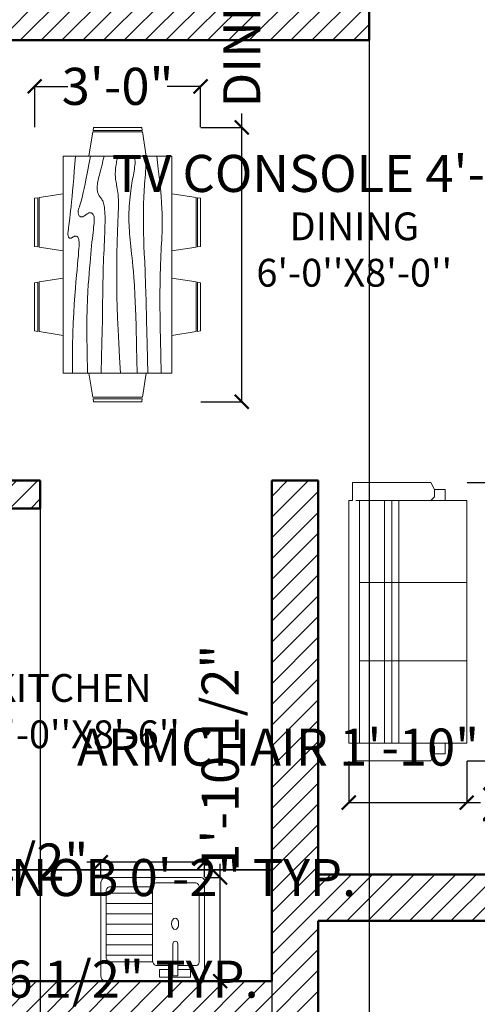
# Model space of a CAD drawing. Units: inches. Extents: x 1945 to 2401, y 1770 to 2289.
# Tile 3 of 5: x 2078 to 2177, y 1893 to 2105. Entities that reach past the tile are written whole.
import ezdxf

# ---------------------------------------------------------------- set-up
doc = ezdxf.new("R2010")
doc.units = ezdxf.units.IN
for name, color, linetype, lineweight in [('A-ANNO-DIMS', 2, 'Continuous', 18), ('A-AREA-IDEN', 7, 'Continuous', 25), ('A-FLOR-FIXT', 9, 'Continuous', 18), ('A-WALL-PATT', 8, 'Continuous', 13), ('B-FURNITURE', 22, 'Continuous', 18), ('kitchen', 122, 'Continuous', 25), ('Walls', 7, 'Continuous', 50)]:
    doc.layers.add(name, color=color, linetype=linetype, lineweight=lineweight)
doc.styles.get("Standard").update_dxf_attribs({"font": 'arial.ttf'})
doc.dimstyles.get("Standard").update_dxf_attribs({"dimtxt": 8, "dimasz": 3, "dimexe": 0.18, "dimexo": 0.0625, "dimgap": 0.09, "dimtad": 0, "dimdec": 1, "dimzin": 0, "dimdsep": 46, "dimlunit": 4, "dimtxsty": 'Standard', "dimblk": 'ARCHTICK', "dimcen": 0.09, "dimadec": 0, "dimazin": 0, "dimtfac": 1, "dimtdec": 1, "dimtofl": 0, "dimtmove": 0, "dimatfit": 3, "dimfxl": 1, "dimtolj": 1, "dimtzin": 0, "dimarcsym": 0})

# ---------------------------------------------------------------- blocks, each defined once
blk = doc.blocks.new('12PCOU13')
at = {"color": 0, "linetype": 'ByBlock'}
for p, q in [((24, 37), (24, 35)), ((23, 34), (2, 34)), ((3, -34), (3, 34)), ((10, 34), (10, -34)), ((12, 34), (12, -34)), ((14, 34), (14, -34)), ((24, 35), (23, 34)), ((27, 34), (23, 34)), ((33, 11), (3, 11)), ((33, -11), (3, -11)), ((23, -34), (2, -34)), ((27, -34), (23, -34)), ((24, -35), (23, -34)), ((24, -37), (24, -35))]:
    blk.add_line(p, q, dxfattribs=at)
blk.add_lwpolyline([(1, -39), (1, -34), (0, -34), (0, 34), (1, 34), (1, 39), (23, 39), (24, 37), (27, 37), (27, 34), (33, 34), (33, -34), (27, -34), (27, -37), (24, -37), (23, -39)], close=True, dxfattribs=at)
blk = doc.blocks.new('Dining Set - 36 x 72 in.')
for p, q in [((-22, 27.5), (-22.1562, 26.50042)), ((-5.8416, 26.5), (-22.1534, 26.5)), ((-22, 27.5), (-6, 27.5)), ((-5.8437, 26.49966), (-6, 27.5)), ((6, 27.5), (5.8438, 26.50042)), ((22.1584, 26.5), (5.8466, 26.5)), ((6, 27.5), (22, 27.5)), ((22.1563, 26.49966), (22, 27.5)), ((-22.2343, 26.00059), (-23.4847, 17.99762)), ((-22.2304, 26), (-5.7608, 26)), ((-4.5152, 17.99762), (-5.7655, 25.99926)), ((5.7657, 26.00059), (4.5153, 17.99762)), ((5.7696, 26), (22.2392, 26)), ((23.4848, 17.99762), (22.2345, 25.99926)), ((36, 18), (-36, 18)), ((-36, 18), (-36, -18)), ((36, -18), (36, 18)), ((-45.5, 8), (-44.5004, 8.15617)), ((-45.5, 8), (-45.5, -8)), ((-44.5, -8.15843), (-44.5, 8.15338)), ((-44.0006, 8.23428), (-35.9976, 9.48474)), ((-44, 8.23041), (-44, -8.23915)), ((44.0006, 8.23428), (35.9976, 9.48474)), ((44, 8.23041), (44, -8.23915)), ((44.5, -8.15843), (44.5, 8.15338)), ((45.5, 8), (44.5005, 8.15617)), ((45.5, 8), (45.5, -8)), ((-44.4997, -8.15631), (-45.5, -8)), ((-35.9976, -9.48476), (-43.9993, -8.2345)), ((35.9976, -9.48476), (43.9993, -8.2345)), ((44.4997, -8.15631), (45.5, -8)), ((-36, -18), (36, -18)), ((-22.2343, -26.0006), (-23.4847, -17.99762)), ((-4.5152, -17.99762), (-5.7655, -25.99928)), ((5.7657, -26.0006), (4.5153, -17.99762)), ((23.4848, -17.99762), (22.2345, -25.99928)), ((-22.2304, -26), (-5.7608, -26)), ((5.7696, -26), (22.2392, -26)), ((-22, -27.5), (-22.1562, -26.50044)), ((-5.8416, -26.5), (-22.1534, -26.5)), ((-22, -27.5), (-6, -27.5)), ((-5.8437, -26.49967), (-6, -27.5)), ((6, -27.5), (5.8438, -26.50044)), ((22.1584, -26.5), (5.8466, -26.5)), ((6, -27.5), (22, -27.5)), ((22.1563, -26.49967), (22, -27.5))]:
    blk.add_line(p, q)
for points in [[(-36, 15), (-31.1772, 14.97754), (-26.8079, 14.91406), (-22.8538, 14.81543), (-19.276, 14.6875), (-16.0362, 14.53613), (-13.0957, 14.36718), (-10.4159, 14.18652), (-7.9583, 14), (-5.6904, 13.81315), (-3.6035, 13.63021), (-1.6954, 13.45508), (0.0365, 13.29166), (1.5945, 13.14388), (2.9811, 13.01562), (4.1988, 12.9108), (5.25, 12.83333), (6.1393, 12.78613), (6.8802, 12.76823), (7.4883, 12.77767), (7.9792, 12.8125), (8.3685, 12.87077), (8.6719, 12.95052), (8.9049, 13.0498), (9.0833, 13.16666), (9.2205, 13.29899), (9.3216, 13.44401), (9.3895, 13.59879), (9.4271, 13.76041), (9.4373, 13.92594), (9.4232, 14.09245), (9.3875, 14.257), (9.3333, 14.41666), (9.2638, 14.56917), (9.1836, 14.71484), (9.0975, 14.85465), (9.0104, 14.98958), (8.9272, 15.1206), (8.8529, 15.2487), (8.7922, 15.37483), (8.75, 15.5), (8.7305, 15.62467), (8.7344, 15.74739), (8.7617, 15.86621), (8.8125, 15.97916), (8.8867, 16.08431), (8.9844, 16.17968), (9.1055, 16.26334), (9.25, 16.33333), (9.4189, 16.38802), (9.6172, 16.42708), (9.8506, 16.45052), (10.125, 16.45833), (10.4463, 16.45052), (10.8203, 16.42708), (11.2529, 16.38802), (11.75, 16.33333), (12.3184, 16.26318), (12.9694, 16.17838), (13.7151, 16.07991), (14.5677, 15.96875), (15.5395, 15.84586), (16.6426, 15.71224), (17.8893, 15.56884), (19.2917, 15.41666), (20.859, 15.25667), (22.5879, 15.08984), (24.4721, 14.91715), (26.5052, 14.73958), (28.6809, 14.5581), (30.9929, 14.3737), (33.4347, 14.18733), (36, 14)], [(-36, 10), (-28.9766, 10.14274), (-23.1725, 10.20442), (-18.4241, 10.19775), (-14.5677, 10.13541), (-11.4399, 10.03011), (-8.877, 9.89453), (-6.7154, 9.74137), (-4.7917, 9.58333), (-2.9698, 9.43082), (-1.2246, 9.28515), (0.4415, 9.14534), (2.026, 9.01041), (3.5266, 8.87939), (4.9408, 8.7513), (6.266, 8.62516), (7.5, 8.5), (8.6411, 8.37549), (9.6914, 8.2539), (10.6538, 8.13818), (11.5312, 8.03125), (12.3267, 7.93603), (13.043, 7.85547), (13.6831, 7.79248), (14.25, 7.75), (14.7471, 7.7303), (15.1797, 7.73307), (15.5537, 7.75732), (15.875, 7.80208), (16.1494, 7.86637), (16.3828, 7.94922), (16.5811, 8.04964), (16.75, 8.16666), (16.8944, 8.29915), (17.0143, 8.44531), (17.1089, 8.60319), (17.1771, 8.77083), (17.218, 8.94629), (17.2305, 9.1276), (17.2137, 9.31282), (17.1667, 9.5), (17.0895, 9.6875), (16.987, 9.875), (16.8649, 10.0625), (16.7292, 10.25), (16.5856, 10.4375), (16.4401, 10.625), (16.2985, 10.8125), (16.1667, 11), (16.05, 11.18733), (15.9518, 11.3737), (15.8752, 11.5581), (15.8229, 11.73958), (15.798, 11.91715), (15.8034, 12.08984), (15.842, 12.25667), (15.9167, 12.41666), (16.0295, 12.56836), (16.1784, 12.70833), (16.3605, 12.83268), (16.5729, 12.9375), (16.8127, 13.01888), (17.0768, 13.07291), (17.3625, 13.0957), (17.6667, 13.08333), (17.9894, 13.03312), (18.3418, 12.94726), (18.7382, 12.82918), (19.1927, 12.68229), (19.7195, 12.51001), (20.3327, 12.31575), (21.0465, 12.10294), (21.875, 11.875), (22.8357, 11.63354), (23.959, 11.37304), (25.2786, 11.08618), (26.8282, 10.76562), (28.6414, 10.40405), (30.752, 9.99414), (33.1936, 9.52856), (36, 9)], [(-36, 5.5), (-30.7157, 5.3348), (-26.069, 5.20963), (-21.9946, 5.11767), (-18.4271, 5.05208), (-15.3009, 5.00602), (-12.5508, 4.97265), (-10.1112, 4.94515), (-7.9167, 4.91666), (-5.909, 4.88167), (-4.0586, 4.83984), (-2.3429, 4.79215), (-0.7396, 4.73958), (0.7739, 4.6831), (2.22, 4.6237), (3.6213, 4.56233), (5, 4.5), (6.373, 4.43782), (7.7344, 4.3776), (9.0723, 4.32129), (10.375, 4.27083), (11.6309, 4.22819), (12.8281, 4.19531), (13.9551, 4.17415), (15, 4.16666), (15.954, 4.17448), (16.819, 4.19791), (17.6001, 4.23698), (18.3021, 4.29166), (18.9299, 4.36198), (19.4883, 4.44791), (19.9823, 4.54948), (20.4167, 4.66666), (20.7969, 4.79899), (21.1302, 4.94401), (21.4245, 5.09879), (21.6875, 5.26041), (21.9271, 5.42594), (22.1511, 5.59245), (22.3672, 5.757), (22.5834, 5.91666), (22.8065, 6.06868), (23.0404, 6.21093), (23.2879, 6.34147), (23.5521, 6.45833), (23.8358, 6.55957), (24.142, 6.64323), (24.4735, 6.70735), (24.8334, 6.75), (25.2235, 6.76969), (25.642, 6.76692), (26.0858, 6.74267), (26.5521, 6.69791), (27.0379, 6.63362), (27.5404, 6.55078), (28.0565, 6.45036), (28.5834, 6.33333), (29.1242, 6.19987), (29.7071, 6.04687), (30.3661, 5.87044), (31.1354, 5.66666), (32.0493, 5.43164), (33.142, 5.16146), (34.4475, 4.85221), (36, 4.5)], [(-36, -1), (-30.7915, -0.6591), (-26.0195, -0.38216), (-21.6519, -0.16284), (-17.6563, 0.00521), (-14.0005, 0.12833), (-10.6523, 0.21289), (-7.5796, 0.26522), (-4.75, 0.29166), (-2.134, 0.29793), (0.2878, 0.28711), (2.5317, 0.26163), (4.6146, 0.22396), (6.5529, 0.17651), (8.3633, 0.12174), (10.0623, 0.06209), (11.6667, 0), (13.1899, -0.06201), (14.6341, -0.1211), (15.9982, -0.17432), (17.2813, -0.21875), (18.4823, -0.25147), (19.6003, -0.26953), (20.6343, -0.27002), (21.5834, -0.25), (22.4481, -0.20768), (23.2357, -0.14584), (23.9549, -0.06836), (24.6146, 0.02083), (25.2235, 0.11784), (25.7904, 0.21875), (26.3241, 0.31966), (26.8334, 0.41666), (27.3265, 0.50618), (27.8099, 0.58593), (28.2894, 0.65397), (28.7709, 0.70833), (29.2601, 0.74707), (29.763, 0.76823), (30.2855, 0.76985), (30.8334, 0.75), (31.4088, 0.70784), (31.9994, 0.64713), (32.589, 0.57275), (33.1615, 0.48958), (33.7008, 0.4025), (34.1908, 0.3164), (34.6153, 0.23616), (34.9584, 0.16666), (35.2099, 0.11165), (35.3848, 0.07031), (35.504, 0.04069), (35.5886, 0.02083), (35.6594, 0.00879), (35.7377, 0.0026), (35.8442, 0.00032), (36, 0)], [(-36, -6.5), (-27.1843, -6.31267), (-20.084, -6.1263), (-14.469, -5.9419), (-10.1094, -5.76042), (-6.7752, -5.58285), (-4.2363, -5.41016), (-2.2629, -5.24333), (-0.625, -5.08334), (0.8708, -4.93099), (2.2715, -4.78646), (3.5872, -4.64974), (4.8281, -4.52084), (6.0046, -4.39974), (7.127, -4.28646), (8.2053, -4.18099), (9.25, -4.08334), (10.2705, -3.99382), (11.2734, -3.91407), (12.2647, -3.84603), (13.25, -3.79167), (14.2354, -3.75293), (15.2266, -3.73177), (16.2295, -3.73015), (17.25, -3.75), (18.2912, -3.79248), (19.3451, -3.85547), (20.4009, -3.93604), (21.4479, -4.03125), (22.4754, -4.13819), (23.4727, -4.25391), (24.4289, -4.37549), (25.3334, -4.5), (26.1785, -4.62492), (26.9694, -4.74935), (27.7145, -4.87281), (28.4219, -4.99479), (29.1, -5.11483), (29.7572, -5.23242), (30.4016, -5.34709), (31.0417, -5.45834), (31.6837, -5.56437), (32.3262, -5.65821), (32.9658, -5.73153), (33.599, -5.77604), (34.2224, -5.78345), (34.8327, -5.74545), (35.4264, -5.65373), (36, -5.5)], [(-36, -10), (-26.4022, -9.81299), (-18.4675, -9.62891), (-11.9839, -9.45069), (-6.7396, -9.28125), (-2.5226, -9.12354), (0.8789, -8.98047), (3.6769, -8.85498), (6.0833, -8.75), (8.2767, -8.66765), (10.3021, -8.60677), (12.1712, -8.56543), (13.8958, -8.54167), (15.4876, -8.53353), (16.9583, -8.53907), (18.3197, -8.55632), (19.5834, -8.58334), (20.7616, -8.61841), (21.8685, -8.66081), (22.9188, -8.71004), (23.9271, -8.76563), (24.9081, -8.82707), (25.8763, -8.89388), (26.8465, -8.96558), (27.8334, -9.04167), (28.8474, -9.12118), (29.8828, -9.20117), (30.93, -9.27824), (31.9792, -9.34896), (33.0205, -9.40991), (34.0443, -9.45768), (35.0407, -9.48885), (36, -9.5)], [(-36, -14.5), (-30.0881, -14.33513), (-25.0332, -14.21224), (-20.7312, -14.12647), (-17.0781, -14.07292), (-13.97, -14.04671), (-11.3027, -14.04297), (-8.9724, -14.05681), (-6.875, -14.08334), (-4.9224, -14.11833), (-3.0905, -14.16016), (-1.3709, -14.20785), (0.2448, -14.26042), (1.7647, -14.3169), (3.1973, -14.3763), (4.5507, -14.43767), (5.8333, -14.5), (7.0554, -14.5621), (8.235, -14.62175), (9.3922, -14.67652), (10.5469, -14.72396), (11.7192, -14.76164), (12.929, -14.78711), (14.1965, -14.79794), (15.5417, -14.79167), (16.9933, -14.76424), (18.6152, -14.70508), (20.4804, -14.60197), (22.6615, -14.44271), (25.2312, -14.21509), (28.2624, -13.9069), (31.8277, -13.50594), (36, -13)]]:
    blk.add_lwpolyline(points)
blk = doc.blocks.new('S_SINK12')
for p, q in [((0.25, 0.45), (0.25, 0.0004)), ((0.35, 0.45), (0.35, 0.0004)), ((0.45, 0.45), (0.45, 0.0004)), ((0.55, 0.45), (0.55, 0.0004)), ((0.65, 0.45), (0.65, 0.0004)), ((0.75, 0.45), (0.75, 0.0004)), ((0.85, 0.45), (0.85, 0.0004))]:
    blk.add_line(p, q)
for points in [[(0, -0.4688), (0, 0.4688, -0.310961), (0.05, 0.4998), (0.95, 0.4998, -0.310466), (1, 0.4686), (1, -0.4688, -0.414214), (0.9687, -0.5), (0.05, -0.5002, -0.309971)], [(0.4997, -0.2171), (0.5033, -0.2291, 0.107136), (0.5156, -0.241, 0.076468), (0.5341, -0.249), (0.5538, -0.2509), (0.5755, -0.2481, 0.076468), (0.5921, -0.241, 0.107136), (0.6044, -0.2291), (0.608, -0.2171), (0.6044, -0.2051, 0.107136), (0.5921, -0.1931, 0.076468), (0.5755, -0.186), (0.5538, -0.1832), (0.5322, -0.186, 0.076468), (0.5156, -0.1931, 0.107136), (0.5033, -0.2051)], [(0.0516, -0.1954), (0.0516, -0.242), (0.3617, -0.242, 1), (0.3617, -0.1954)]]:
    blk.add_lwpolyline(points, format="xyb", close=True)
for points in [[(0.1851, -0.001), (0.1851, 0.4188, -0.310466), (0.2351, 0.45), (0.8621, 0.45, -0.310466), (0.9121, 0.4188), (0.9121, -0.0005, -0.310466)], [(0.15, -0.1954), (0.15, -0.0308, -0.310466), (0.2, 0.0004), (0.9, 0.0004, -0.310466), (0.95, -0.0308), (0.95, -0.4189, -0.310466), (0.9, -0.4502), (0.2, -0.4502), (0.1799, -0.4479, -0.071009), (0.1646, -0.4419, -0.106323), (0.1531, -0.4318), (0.1499, -0.422), (0.1508, -0.4192)]]:
    blk.add_lwpolyline(points, format="xyb")
for points in [[(0.1136, -0.242), (0.1136, -0.3644), (0.0386, -0.3644), (0.0386, -0.0644), (0.1136, -0.0644), (0.1136, -0.1954)], [(0.15, -0.4189), (0.15, -0.242)]]:
    blk.add_lwpolyline(points)
blk = doc.blocks.new('_ArchTick')
at = {"color": 0, "linetype": 'ByBlock', "const_width": 0.15}
blk.add_lwpolyline([(-0.5, -0.5), (0.5, 0.5)], dxfattribs=at)
blk = doc.blocks.new('*D30')
at = {"layer": 'A-ANNO-DIMS', "color": 0, "lineweight": -2, "transparency": 16777216}
for p, q in [((2052.64, 1899.41), (2052.64, 1898.29)), ((2059.37, 1899.41), (2059.37, 1898.29)), ((2052.64, 1898.47), (2059.37, 1898.47)), ((2059.37, 1898.47), (2062.37, 1898.47))]:
    blk.add_line(p, q, dxfattribs=at)
at = {"layer": 'Defpoints', "color": 0, "transparency": 16777216}
for p in [(2052.64, 1899.48), (2059.37, 1899.48), (2059.37, 1898.47)]:
    blk.add_point(p, dxfattribs=at)
at = {"layer": 'A-ANNO-DIMS', "color": 0, "lineweight": -2, "transparency": 16777216, "xscale": 3, "yscale": 3, "zscale": 3, "rotation": 180}
blk.add_blockref('_ArchTick', (2052.64, 1898.47), dxfattribs=at)
at = {"layer": 'A-ANNO-DIMS', "color": 0, "lineweight": -2, "transparency": 16777216, "xscale": 3, "yscale": 3, "zscale": 3}
blk.add_blockref('_ArchTick', (2059.37, 1898.47), dxfattribs=at)
at = {"layer": 'A-ANNO-DIMS', "color": 0, "transparency": 16777216, "insert": (2096.16, 1898.47), "char_height": 8, "attachment_point": 5}
blk.add_mtext('\\A1;0\'-6 1/2" TYP.', dxfattribs=at)
blk = doc.blocks.new('*D31')
at = {"layer": 'A-ANNO-DIMS', "color": 0, "lineweight": -2, "transparency": 16777216}
for p, q in [((2063.65, 1920.15), (2063.65, 1920.56)), ((2063.65, 1920.38), (2065.6, 1920.38)), ((2065.6, 1920.15), (2065.6, 1920.56)), ((2065.6, 1920.38), (2068.6, 1920.38))]:
    blk.add_line(p, q, dxfattribs=at)
at = {"layer": 'Defpoints', "color": 0, "transparency": 16777216}
for p in [(2065.6, 1920.38), (2063.65, 1920.08), (2065.6, 1920.08)]:
    blk.add_point(p, dxfattribs=at)
at = {"layer": 'A-ANNO-DIMS', "color": 0, "lineweight": -2, "transparency": 16777216, "xscale": 3, "yscale": 3, "zscale": 3, "rotation": 180}
blk.add_blockref('_ArchTick', (2063.65, 1920.38), dxfattribs=at)
at = {"layer": 'A-ANNO-DIMS', "color": 0, "lineweight": -2, "transparency": 16777216, "xscale": 3, "yscale": 3, "zscale": 3}
blk.add_blockref('_ArchTick', (2065.6, 1920.38), dxfattribs=at)
at = {"layer": 'A-ANNO-DIMS', "color": 0, "transparency": 16777216, "insert": (2110.28, 1920.38), "char_height": 8, "attachment_point": 5}
blk.add_mtext('\\A1;KNOB 0\'-2" TYP.', dxfattribs=at)
blk = doc.blocks.new('*D37')
at = {"layer": 'A-ANNO-DIMS', "color": 0, "lineweight": -2, "transparency": 16777216}
for p, q in [((2183.86, 2005.62), (2183.86, 2008.62)), ((2174.92, 2005.62), (2184.04, 2005.62)), ((2183.86, 1945.56), (2183.86, 2005.62)), ((2174.92, 1945.56), (2184.04, 1945.56))]:
    blk.add_line(p, q, dxfattribs=at)
at = {"layer": 'Defpoints', "color": 0, "transparency": 16777216}
for p in [(2174.85, 2005.62), (2183.86, 2005.62), (2174.85, 1945.56)]:
    blk.add_point(p, dxfattribs=at)
at = {"layer": 'A-ANNO-DIMS', "color": 0, "lineweight": -2, "transparency": 16777216, "xscale": 3, "yscale": 3, "zscale": 3}
for p, rotation in [((2183.86, 2005.62), 90), ((2183.86, 1945.56), 270)]:
    blk.add_blockref('_ArchTick', p, dxfattribs=dict(at, rotation=rotation))
at = {"layer": 'A-ANNO-DIMS', "color": 0, "transparency": 16777216, "insert": (2183.86, 2049.84), "char_height": 8, "attachment_point": 5, "rotation": 90}
blk.add_mtext('\\A1;SOFA 5\'-0" TYP.', dxfattribs=at)
blk = doc.blocks.new('*D38')
at = {"layer": 'A-ANNO-DIMS', "color": 0, "lineweight": -2, "transparency": 16777216}
for p, q in [((2149.44, 1945.5), (2149.44, 1936.37)), ((2174.85, 1945.5), (2174.85, 1936.37)), ((2149.44, 1936.55), (2174.85, 1936.55)), ((2174.85, 1936.55), (2177.85, 1936.55))]:
    blk.add_line(p, q, dxfattribs=at)
at = {"layer": 'Defpoints', "color": 0, "transparency": 16777216}
for p in [(2149.44, 1945.56), (2174.85, 1945.56), (2174.85, 1936.55)]:
    blk.add_point(p, dxfattribs=at)
at = {"layer": 'A-ANNO-DIMS', "color": 0, "lineweight": -2, "transparency": 16777216, "xscale": 3, "yscale": 3, "zscale": 3, "rotation": 180}
blk.add_blockref('_ArchTick', (2149.44, 1936.55), dxfattribs=at)
at = {"layer": 'A-ANNO-DIMS', "color": 0, "lineweight": -2, "transparency": 16777216, "xscale": 3, "yscale": 3, "zscale": 3}
blk.add_blockref('_ArchTick', (2174.85, 1936.55), dxfattribs=at)
at = {"layer": 'A-ANNO-DIMS', "color": 0, "transparency": 16777216, "insert": (2211.71, 1936.55), "char_height": 8, "attachment_point": 5}
blk.add_mtext('\\A1;2\'-1 1/2" TYP.', dxfattribs=at)
blk = doc.blocks.new('*D39')
at = {"layer": 'A-ANNO-DIMS', "color": 0, "lineweight": -2, "transparency": 16777216}
for p, q in [((2208.72, 1948.53), (2205.72, 1948.53)), ((2208.72, 1945.26), (2208.72, 1948.71)), ((2230.95, 1948.53), (2208.72, 1948.53)), ((2230.95, 1945.26), (2230.95, 1948.71))]:
    blk.add_line(p, q, dxfattribs=at)
at = {"layer": 'Defpoints', "color": 0, "transparency": 16777216}
for p in [(2208.72, 1948.53), (2208.72, 1945.2), (2230.95, 1945.2)]:
    blk.add_point(p, dxfattribs=at)
at = {"layer": 'A-ANNO-DIMS', "color": 0, "lineweight": -2, "transparency": 16777216, "xscale": 3, "yscale": 3, "zscale": 3, "rotation": 180}
blk.add_blockref('_ArchTick', (2208.72, 1948.53), dxfattribs=at)
at = {"layer": 'A-ANNO-DIMS', "color": 0, "lineweight": -2, "transparency": 16777216, "xscale": 3, "yscale": 3, "zscale": 3}
blk.add_blockref('_ArchTick', (2230.95, 1948.53), dxfattribs=at)
at = {"layer": 'A-ANNO-DIMS', "color": 0, "transparency": 16777216, "insert": (2146.55, 1948.53), "char_height": 8, "attachment_point": 5}
blk.add_mtext('\\A1;ARMCHAIR 1\'-10" TYP.', dxfattribs=at)
blk = doc.blocks.new('*D43')
at = {"layer": 'A-ANNO-DIMS', "color": 0, "lineweight": -2, "transparency": 16777216}
for p, q in [((2060.9, 2111.04), (2064.52, 2111.04)), ((2064.34, 2111.04), (2064.34, 2087.72)), ((2060.9, 2087.72), (2064.52, 2087.72)), ((2064.34, 2087.72), (2064.34, 2084.72))]:
    blk.add_line(p, q, dxfattribs=at)
at = {"layer": 'Defpoints', "color": 0, "transparency": 16777216}
for p in [(2060.84, 2111.04), (2060.84, 2087.72), (2064.34, 2087.72)]:
    blk.add_point(p, dxfattribs=at)
at = {"layer": 'A-ANNO-DIMS', "color": 0, "lineweight": -2, "transparency": 16777216, "xscale": 3, "yscale": 3, "zscale": 3}
for p, rotation in [((2064.34, 2111.04), 90), ((2064.34, 2087.72), 270)]:
    blk.add_blockref('_ArchTick', p, dxfattribs=dict(at, rotation=rotation))
at = {"layer": 'A-ANNO-DIMS', "color": 0, "transparency": 16777216, "insert": (2064.34, 2026.98), "char_height": 8, "attachment_point": 5, "rotation": 90}
blk.add_mtext('\\A1;BATH DOOR 1\'-11 1/2"', dxfattribs=at)
blk = doc.blocks.new('*D53')
at = {"layer": 'A-ANNO-DIMS', "color": 0, "lineweight": -2, "transparency": 16777216}
for p, q in [((2126.35, 2082.22), (2126.35, 2085.22)), ((2117.54, 2082.22), (2126.53, 2082.22)), ((2126.35, 2023.05), (2126.35, 2082.22)), ((2117.54, 2023.05), (2126.53, 2023.05))]:
    blk.add_line(p, q, dxfattribs=at)
at = {"layer": 'Defpoints', "color": 0, "transparency": 16777216}
for p in [(2117.47, 2082.22), (2126.35, 2082.22), (2117.47, 2023.05)]:
    blk.add_point(p, dxfattribs=at)
at = {"layer": 'A-ANNO-DIMS', "color": 0, "lineweight": -2, "transparency": 16777216, "xscale": 3, "yscale": 3, "zscale": 3}
for p, rotation in [((2126.35, 2082.22), 90), ((2126.35, 2023.05), 270)]:
    blk.add_blockref('_ArchTick', p, dxfattribs=dict(at, rotation=rotation))
at = {"layer": 'A-ANNO-DIMS', "color": 0, "transparency": 16777216, "insert": (2126.35, 2132.38), "char_height": 8, "attachment_point": 5, "rotation": 90}
blk.add_mtext('\\A1;DINING SET 4\'-11"', dxfattribs=at)
blk = doc.blocks.new('*D54')
at = {"layer": 'A-ANNO-DIMS', "color": 0, "lineweight": -2, "transparency": 16777216}
for p, q in [((2081.71, 2082.28), (2081.71, 2091.27)), ((2081.71, 2091.09), (2088.87, 2091.09)), ((2117.47, 2091.09), (2110.31, 2091.09)), ((2117.47, 2082.28), (2117.47, 2091.27))]:
    blk.add_line(p, q, dxfattribs=at)
at = {"layer": 'Defpoints', "color": 0, "transparency": 16777216}
for p in [(2081.71, 2091.09), (2081.71, 2082.22), (2117.47, 2082.22)]:
    blk.add_point(p, dxfattribs=at)
at = {"layer": 'A-ANNO-DIMS', "color": 0, "lineweight": -2, "transparency": 16777216, "xscale": 3, "yscale": 3, "zscale": 3, "rotation": 180}
blk.add_blockref('_ArchTick', (2081.71, 2091.09), dxfattribs=at)
at = {"layer": 'A-ANNO-DIMS', "color": 0, "lineweight": -2, "transparency": 16777216, "xscale": 3, "yscale": 3, "zscale": 3}
blk.add_blockref('_ArchTick', (2117.47, 2091.09), dxfattribs=at)
at = {"layer": 'A-ANNO-DIMS', "color": 0, "transparency": 16777216, "insert": (2099.59, 2091.09), "char_height": 8, "attachment_point": 5}
blk.add_mtext('\\A1;3\'-0"', dxfattribs=at)
blk = doc.blocks.new('*D55')
at = {"layer": 'A-ANNO-DIMS', "color": 0, "lineweight": -2, "transparency": 16777216}
for p, q in [((2195.59, 2080.82), (2195.59, 2072.12)), ((2252.8, 2080.82), (2252.8, 2072.12)), ((2195.59, 2072.3), (2192.59, 2072.3)), ((2252.8, 2072.3), (2195.59, 2072.3))]:
    blk.add_line(p, q, dxfattribs=at)
at = {"layer": 'Defpoints', "color": 0, "transparency": 16777216}
for p in [(2195.59, 2080.88), (2252.8, 2080.88), (2195.59, 2072.3)]:
    blk.add_point(p, dxfattribs=at)
at = {"layer": 'A-ANNO-DIMS', "color": 0, "lineweight": -2, "transparency": 16777216, "xscale": 3, "yscale": 3, "zscale": 3, "rotation": 180}
blk.add_blockref('_ArchTick', (2195.59, 2072.3), dxfattribs=at)
at = {"layer": 'A-ANNO-DIMS', "color": 0, "lineweight": -2, "transparency": 16777216, "xscale": 3, "yscale": 3, "zscale": 3}
blk.add_blockref('_ArchTick', (2252.8, 2072.3), dxfattribs=at)
at = {"layer": 'A-ANNO-DIMS', "color": 0, "transparency": 16777216, "insert": (2144.19, 2072.3), "char_height": 8, "attachment_point": 5}
blk.add_mtext('\\A1;TV CONSOLE 4\'-9"', dxfattribs=at)
blk = doc.blocks.new('*D57')
at = {"layer": 'A-ANNO-DIMS', "color": 0, "lineweight": -2, "transparency": 16777216}
for p, q in [((2095.97, 1923.73), (2092.97, 1923.73)), ((2095.97, 1920.44), (2095.97, 1923.91)), ((2118.35, 1923.73), (2095.97, 1923.73)), ((2118.35, 1920.44), (2118.35, 1923.91))]:
    blk.add_line(p, q, dxfattribs=at)
at = {"layer": 'Defpoints', "color": 0, "transparency": 16777216}
for p in [(2095.97, 1923.73), (2095.97, 1920.38), (2118.35, 1920.38)]:
    blk.add_point(p, dxfattribs=at)
at = {"layer": 'A-ANNO-DIMS', "color": 0, "lineweight": -2, "transparency": 16777216, "xscale": 3, "yscale": 3, "zscale": 3, "rotation": 180}
blk.add_blockref('_ArchTick', (2095.97, 1923.73), dxfattribs=at)
at = {"layer": 'A-ANNO-DIMS', "color": 0, "lineweight": -2, "transparency": 16777216, "xscale": 3, "yscale": 3, "zscale": 3}
blk.add_blockref('_ArchTick', (2118.35, 1923.73), dxfattribs=at)
at = {"layer": 'A-ANNO-DIMS', "color": 0, "transparency": 16777216, "insert": (2055.24, 1923.73), "char_height": 8, "attachment_point": 5}
blk.add_mtext('\\A1;SINK 1\'-10 1/2"', dxfattribs=at)
blk = doc.blocks.new('*D58')
at = {"layer": 'A-ANNO-DIMS', "color": 0, "lineweight": -2, "transparency": 16777216}
for p, q in [((2121.7, 1920.38), (2121.7, 1923.38)), ((2118.41, 1920.38), (2121.88, 1920.38)), ((2121.7, 1898.04), (2121.7, 1920.38)), ((2118.41, 1898.04), (2121.88, 1898.04))]:
    blk.add_line(p, q, dxfattribs=at)
at = {"layer": 'Defpoints', "color": 0, "transparency": 16777216}
for p in [(2118.35, 1920.38), (2121.7, 1920.38), (2118.35, 1898.04)]:
    blk.add_point(p, dxfattribs=at)
at = {"layer": 'A-ANNO-DIMS', "color": 0, "lineweight": -2, "transparency": 16777216, "xscale": 3, "yscale": 3, "zscale": 3}
for p, rotation in [((2121.7, 1920.38), 90), ((2121.7, 1898.04), 270)]:
    blk.add_blockref('_ArchTick', p, dxfattribs=dict(at, rotation=rotation))
at = {"layer": 'A-ANNO-DIMS', "color": 0, "transparency": 16777216, "insert": (2121.7, 1946.15), "char_height": 8, "attachment_point": 5, "rotation": 90}
blk.add_mtext('\\A1;1\'-10 1/2"', dxfattribs=at)
blk = doc.blocks.new('*D65')
at = {"layer": 'A-ANNO-DIMS', "color": 0, "lineweight": -2, "transparency": 16777216}
for p, q in [((2142.84, 1910.98), (2142.84, 1781.89)), ((2179.42, 1910.98), (2179.42, 1781.89)), ((2142.84, 1782.07), (2179.42, 1782.07)), ((2179.42, 1782.07), (2182.42, 1782.07))]:
    blk.add_line(p, q, dxfattribs=at)
at = {"layer": 'Defpoints', "color": 0, "transparency": 16777216}
for p in [(2142.84, 1911.04), (2179.42, 1911.04), (2179.42, 1782.07)]:
    blk.add_point(p, dxfattribs=at)
at = {"layer": 'A-ANNO-DIMS', "color": 0, "lineweight": -2, "transparency": 16777216, "xscale": 3, "yscale": 3, "zscale": 3, "rotation": 180}
blk.add_blockref('_ArchTick', (2142.84, 1782.07), dxfattribs=at)
at = {"layer": 'A-ANNO-DIMS', "color": 0, "lineweight": -2, "transparency": 16777216, "xscale": 3, "yscale": 3, "zscale": 3}
blk.add_blockref('_ArchTick', (2179.42, 1782.07), dxfattribs=at)
at = {"layer": 'A-ANNO-DIMS', "color": 0, "transparency": 16777216, "insert": (2202.46, 1782.07), "char_height": 8, "attachment_point": 5}
blk.add_mtext('\\A1;3\'-0 1/2"', dxfattribs=at)
blk = doc.blocks.new('*D68')
at = {"layer": 'A-ANNO-DIMS', "color": 0, "lineweight": -2, "transparency": 16777216}
for p, q in [((2132.78, 1922.04), (1978.76, 1922.04)), ((1978.94, 1922.04), (1978.94, 1920.83)), ((1978.94, 1898.04), (1978.94, 1899.25)), ((2132.78, 1898.04), (1978.76, 1898.04))]:
    blk.add_line(p, q, dxfattribs=at)
at = {"layer": 'Defpoints', "color": 0, "transparency": 16777216}
for p in [(1978.94, 1922.04), (2132.84, 1922.04), (2132.84, 1898.04)]:
    blk.add_point(p, dxfattribs=at)
at = {"layer": 'A-ANNO-DIMS', "color": 0, "lineweight": -2, "transparency": 16777216, "xscale": 3, "yscale": 3, "zscale": 3}
for p, rotation in [((1978.94, 1922.04), 90), ((1978.94, 1898.04), 270)]:
    blk.add_blockref('_ArchTick', p, dxfattribs=dict(at, rotation=rotation))
at = {"layer": 'A-ANNO-DIMS', "color": 0, "transparency": 16777216, "insert": (1978.94, 1910.04), "char_height": 8, "attachment_point": 5, "rotation": 90}
blk.add_mtext('\\A1;2\'-0"', dxfattribs=at)
blk = doc.blocks.new('*D69')
at = {"layer": 'A-ANNO-DIMS', "color": 0, "lineweight": -2, "transparency": 16777216}
for p, q in [((2132.84, 2005.98), (2132.84, 1781.89)), ((2082.92, 1999.98), (2082.92, 1781.89)), ((2082.92, 1782.07), (2097, 1782.07)), ((2132.84, 1782.07), (2118.77, 1782.07))]:
    blk.add_line(p, q, dxfattribs=at)
at = {"layer": 'Defpoints', "color": 0, "transparency": 16777216}
for p in [(2132.84, 2006.04), (2082.92, 2000.04), (2132.84, 1782.07)]:
    blk.add_point(p, dxfattribs=at)
at = {"layer": 'A-ANNO-DIMS', "color": 0, "lineweight": -2, "transparency": 16777216, "xscale": 3, "yscale": 3, "zscale": 3, "rotation": 180}
blk.add_blockref('_ArchTick', (2082.92, 1782.07), dxfattribs=at)
at = {"layer": 'A-ANNO-DIMS', "color": 0, "lineweight": -2, "transparency": 16777216, "xscale": 3, "yscale": 3, "zscale": 3}
blk.add_blockref('_ArchTick', (2132.84, 1782.07), dxfattribs=at)
at = {"layer": 'A-ANNO-DIMS', "color": 0, "transparency": 16777216, "insert": (2107.88, 1782.07), "char_height": 8, "attachment_point": 5}
blk.add_mtext('\\A1;4\'-2"', dxfattribs=at)
blk = doc.blocks.new('*D70')
at = {"layer": 'A-ANNO-DIMS', "color": 0, "lineweight": -2, "transparency": 16777216}
for p, q in [((2153.84, 2100.98), (2153.84, 1781.89)), ((2181.84, 2100.98), (2181.84, 1781.89)), ((2153.84, 1782.07), (2157.05, 1782.07)), ((2181.84, 1782.07), (2178.63, 1782.07))]:
    blk.add_line(p, q, dxfattribs=at)
at = {"layer": 'Defpoints', "color": 0, "transparency": 16777216}
for p in [(2153.84, 2101.04), (2181.84, 2101.04), (2181.84, 1782.07)]:
    blk.add_point(p, dxfattribs=at)
at = {"layer": 'A-ANNO-DIMS', "color": 0, "lineweight": -2, "transparency": 16777216, "xscale": 3, "yscale": 3, "zscale": 3, "rotation": 180}
blk.add_blockref('_ArchTick', (2153.84, 1782.07), dxfattribs=at)
at = {"layer": 'A-ANNO-DIMS', "color": 0, "lineweight": -2, "transparency": 16777216, "xscale": 3, "yscale": 3, "zscale": 3}
blk.add_blockref('_ArchTick', (2181.84, 1782.07), dxfattribs=at)
at = {"layer": 'A-ANNO-DIMS', "color": 0, "transparency": 16777216, "insert": (2167.84, 1782.07), "char_height": 8, "attachment_point": 5}
blk.add_mtext('\\A1;2\'-4"', dxfattribs=at)

msp = doc.modelspace()

# ---------------------------------------------------------------- hatches: boundary and pattern name
at = {"layer": 'A-WALL-PATT', "transparency": 33554585}
h = msp.add_hatch(dxfattribs=at)
h.set_pattern_fill('ANSI31', color=256)
h.paths.add_polyline_path([(2142.84, 2006.04), (2132.84, 2006.04), (2132.84, 1898.04), (2012.84, 1898.04), (2012.84, 1888.04), (2142.84, 1888.04), (2142.84, 1911.04), (2179.42, 1911.04), (2179.42, 1921.04), (2142.84, 1921.04)])
h.paths.add_polyline_path([(2269.5, 1921.04), (2239.42, 1921.04), (2239.42, 1911.04), (2269.5, 1911.04)])
h.paths.add_polyline_path([(2332.84, 1981.04), (2322.84, 1981.04), (2322.84, 1921.04), (2311.84, 1921.04), (2311.84, 1911.04), (2322.84, 1911.04), (2322.84, 1817.97), (2332.84, 1817.97)])
h.paths.add_polyline_path([(2012.84, 1931.04), (2002.84, 1931.04), (2002.84, 1806.04), (2142.84, 1806.04), (2142.84, 1816.04), (2012.84, 1816.04)])
h.paths.add_polyline_path([(2012.84, 2000.04), (2082.92, 2000.04), (2082.92, 2006.04), (2066.84, 2006.04), (2066.84, 2101.04), (2142.84, 2101.04), (2153.84, 2101.04), (2153.84, 2111.04), (2142.84, 2111.04), (2142.84, 2118.04), (2132.84, 2118.04), (2132.84, 2111.04), (2060.84, 2111.04), (2060.84, 2006.04), (2012.84, 2006.04), (2012.84, 2026.45), (2002.84, 2026.45), (2002.84, 1967.04), (2012.84, 1967.04)])

# ---------------------------------------------------------------- linework, layer by layer
at = {"layer": 'kitchen'}
msp.add_line((2036.84, 1922.04), (2132.84, 1922.04), dxfattribs=at)
at = {"layer": 'Walls'}
for p, q in [((2153.84, 2111.04), (2153.84, 2101.04)), ((2066.84, 2101.04), (2142.84, 2101.04)), ((2153.84, 2101.04), (2142.84, 2101.04)), ((2066.84, 2006.04), (2082.92, 2006.04)), ((2082.92, 2006.04), (2082.92, 2000.04)), ((2132.84, 2006.04), (2132.84, 1898.04)), ((2132.84, 2006.04), (2142.84, 2006.04)), ((2142.84, 2006.04), (2142.84, 1921.04)), ((2012.84, 2000.04), (2082.92, 2000.04)), ((2142.84, 1921.04), (2271.24, 1921.04)), ((2142.84, 1911.04), (2271.24, 1911.04)), ((2142.84, 1911.04), (2142.84, 1888.04)), ((2012.84, 1898.04), (2132.84, 1898.04))]:
    msp.add_line(p, q, dxfattribs=at)

# ---------------------------------------------------------------- block references
at = {"layer": 'A-FLOR-FIXT', "xscale": 22.33726976405457, "yscale": 22.33726976405457, "zscale": 22.33726976405457, "rotation": 90}
msp.add_blockref('S_SINK12', (2107.15, 1898.04), dxfattribs=at)
at = {"layer": 'B-FURNITURE', "xscale": 0.650215014486131, "yscale": 0.650215014486131, "zscale": 0.650215014486131, "rotation": 90}
msp.add_blockref('Dining Set - 36 x 72 in.', (2099.59, 2052.63), dxfattribs=at)
at = {"layer": 'B-FURNITURE', "xscale": 0.770001005946072, "yscale": 0.770001005946072, "zscale": 0.770001005946072}
msp.add_blockref('12PCOU13', (2149.44, 1975.59), dxfattribs=at)

# ---------------------------------------------------------------- texts
at = {"layer": 'A-AREA-IDEN', "char_height": 6, "attachment_point": 1}
for s, insert in [("\\pxqc;DINING\\P6'-0''X8'-0''", (2124.44, 2063.88)), ("\\pxqc;KITCHEN\\P10'-0''X8'-6''", (2063.47, 1964.29))]:
    msp.add_mtext_dynamic_manual_height_columns(s, width=52.3454, gutter_width=12.5, heights=[0], dxfattribs=dict(at, insert=insert))

# ---------------------------------------------------------------- dimensions: what is measured, and where the dimension line sits
at = {"layer": 'A-ANNO-DIMS'}
for base, p1, p2, angle, text, picture, middle in [((2126.35, 2082.22), (2117.47, 2023.05), (2117.47, 2082.22), 90, 'DINING SET <>', '*D53', (2126.35, 2132.38)), ((2064.34, 2087.72), (2060.84, 2111.04), (2060.84, 2087.72), 270, 'BATH DOOR <>', '*D43', (2064.34, 2026.98)), ((2195.59, 2072.3), (2252.8, 2080.88), (2195.59, 2080.88), 180, 'TV CONSOLE <>', '*D55', (2144.19, 2072.3)), ((2183.86, 2005.62), (2174.85, 1945.56), (2174.85, 2005.62), 90, 'SOFA <> TYP.', '*D37', (2183.86, 2049.84)), ((2208.72, 1948.53), (2230.95, 1945.2), (2208.72, 1945.2), 180, 'ARMCHAIR <> TYP.', '*D39', (2146.55, 1948.53)), ((2095.97, 1923.73), (2118.35, 1920.38), (2095.97, 1920.38), 180, 'SINK <>', '*D57', (2055.24, 1923.73))]:
    dim = msp.add_linear_dim(base=base, p1=p1, p2=p2, angle=angle, text=text, dimstyle='Standard', override={"dimdec": 1, "dimlfac": 1, "dimrnd": 0, "dimzin": 1, "dimdsep": 46, "dimlunit": 4, "dimfrac": 2}, dxfattribs=at)
    dim.commit()
    dim.dimension.update_dxf_attribs({"geometry": picture, "text_midpoint": middle})
for base, p1, p2, picture, middle in [((2181.84, 1782.07), (2153.84, 2101.04), (2181.84, 2101.04), '*D70', (2167.84, 1782.07)), ((2132.84, 1782.07), (2082.92, 2000.04), (2132.84, 2006.04), '*D69', (2107.88, 1782.07)), ((2179.42, 1782.07), (2142.84, 1911.04), (2179.42, 1911.04), '*D65', (2202.46, 1782.07))]:
    dim = msp.add_linear_dim(base=base, p1=p1, p2=p2, dimstyle='Standard', override={"dimdec": 1, "dimlfac": 1, "dimrnd": 0, "dimzin": 1, "dimdsep": 46, "dimlunit": 4, "dimfrac": 2}, dxfattribs=at)
    dim.commit()
    dim.dimension.update_dxf_attribs({"geometry": picture, "text_midpoint": middle})
for base, p1, p2, angle, picture, middle in [((2081.71, 2091.09), (2117.47, 2082.22), (2081.71, 2082.22), 180, '*D54', (2099.59, 2091.09)), ((2121.7, 1920.38), (2118.35, 1898.04), (2118.35, 1920.38), 90, '*D58', (2121.7, 1946.15)), ((1978.94, 1922.04), (2132.84, 1898.04), (2132.84, 1922.04), 90, '*D68', (1978.94, 1910.04))]:
    dim = msp.add_linear_dim(base=base, p1=p1, p2=p2, angle=angle, dimstyle='Standard', override={"dimdec": 1, "dimlfac": 1, "dimrnd": 0, "dimzin": 1, "dimdsep": 46, "dimlunit": 4, "dimfrac": 2}, dxfattribs=at)
    dim.commit()
    dim.dimension.update_dxf_attribs({"geometry": picture, "text_midpoint": middle})
for base, p1, p2, text, picture, middle in [((2174.85, 1936.55), (2149.44, 1945.56), (2174.85, 1945.56), '<> TYP.', '*D38', (2211.71, 1936.55)), ((2065.5978, 1920.3771), (2063.6501, 1920.0849), (2065.5978, 1920.0849), 'KNOB <> TYP.', '*D31', (2110.2813, 1920.3771)), ((2059.37, 1898.47), (2052.64, 1899.48), (2059.37, 1899.48), '<> TYP.', '*D30', (2096.16, 1898.47))]:
    dim = msp.add_linear_dim(base=base, p1=p1, p2=p2, text=text, dimstyle='Standard', override={"dimdec": 1, "dimlfac": 1, "dimrnd": 0, "dimzin": 1, "dimdsep": 46, "dimlunit": 4, "dimfrac": 2}, dxfattribs=at)
    dim.commit()
    dim.dimension.update_dxf_attribs({"geometry": picture, "text_midpoint": middle})

doc.saveas('drawing.dxf')
